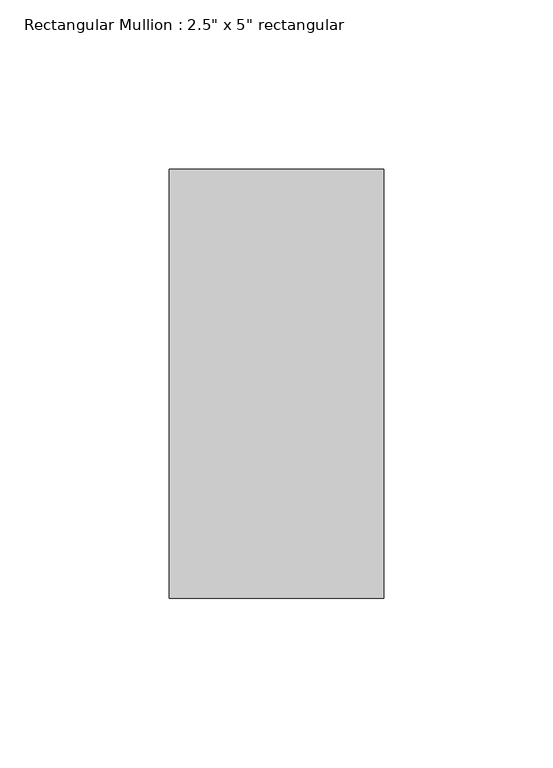
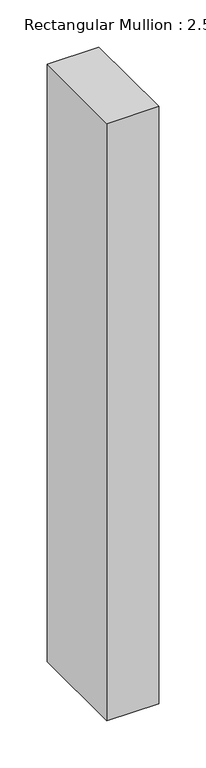
"""IFC4 building model written with IfcOpenShell, lengths in millimetres: member geometry."""

from ifc_helpers import new_model, si_unit, frame, origin, place, context, project, spatial, polyline, outline, extrude, source, transform, mapped, element, save


def member_43aa0f4e(model_context):
    return source(origin(), model_context, "Body", "SweptSolid", [
        extrude(outline(polyline([(0.0, 63.5), (0.0, -63.5), (-63.5, -63.5), (-63.5, 63.5), (0.0, 63.5)])), frame((0.0, 0.0, -775.2709318), z_axis=(0.0, 0.0, 1.0), x_axis=(1.0, 0.0, 0.0)), (0.0, 0.0, 1.0), 775.2709318),
    ])


if __name__ == "__main__":
    model = new_model("IFC4")
    model_context = context("Model", 3, world=origin())
    ifc_project = project(units=[si_unit("LENGTHUNIT", "METRE", prefix="MILLI")], contexts=[model_context])
    site = spatial("IfcSite", under=ifc_project)
    building = spatial("IfcBuilding", under=site)
    placement = place(None, origin())
    member_shape = member_43aa0f4e(model_context)
    element("IfcMember", 1, ObjectType="Rectangular Mullion : 2.5\" x 5\" rectangular", at=placement, inside=building, context=model_context, shape_type="MappedRepresentation", body=[
        mapped(member_shape, transform((0.0, 0.0, 0.0), x_axis=(1.0, 0.0, 0.0), y_axis=(0.0, 1.0, 0.0), z_axis=(0.0, 0.0, 1.0))),
    ])
    save(model, "model.ifc")

# Revit data of these elements
# Type "Rectangular Mullion : 2.5\" x 5\" rectangular"
#   built-in parameter 1007304 = 0.416667 (stored number, unit not read)
#   built-in parameter 1007301 = 0.104167 (stored number, unit not read)
#   built-in parameter 1007300 = 0.104167 (stored number, unit not read)
# Element 1 (IfcMember, "Rectangular Mullion : 2.5\" x 5\" rectangular")
#   Materials on its faces: "Aluminum"
# Materials
#   "Aluminum": class "Metal", colour RGB 247 247 247, transparency 0, Description = "Aluminum 6061", Cost = 0
